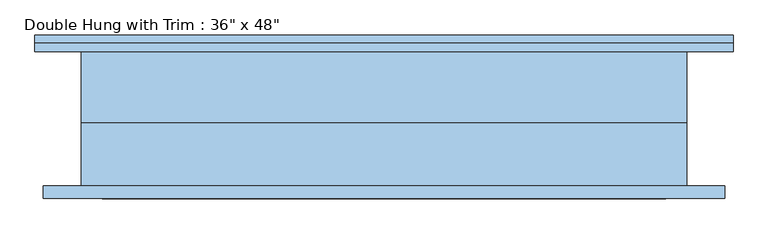
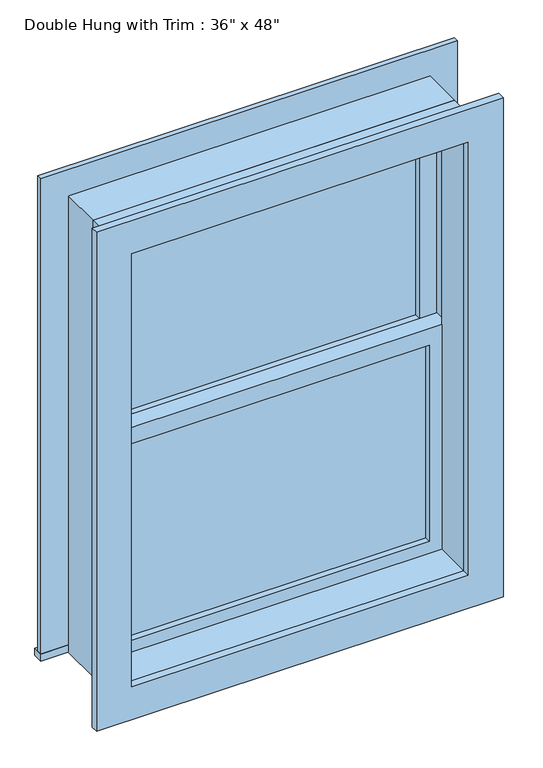
"""IFC4 building model written with IfcOpenShell, lengths in millimetres: window geometry."""

from ifc_helpers import new_model, si_unit, frame, origin, place, context, project, spatial, polyline, outline, extrude, source, transform, mapped, element, save


def window_31198920(model_context):
    return source(origin(), model_context, "Body", "SweptSolid", [
        extrude(outline(polyline([(-393.7, 22.225), (393.7, 22.225), (393.7, 9.525), (-393.7, 9.525), (-393.7, 22.225)])), frame((0.0, 0.0, 977.9), z_axis=(0.0, 0.0, 1.0), x_axis=(1.0, 0.0, 0.0)), (0.0, 0.0, 1.0), 523.875),
        extrude(outline(polyline([(1546.225, -438.15), (933.45, -438.15), (933.45, 438.15), (1546.225, 438.15), (1546.225, -438.15)]), holes=[polyline([(1501.775, -393.7), (1501.775, 393.7), (977.9, 393.7), (977.9, -393.7), (1501.775, -393.7)])]), frame((0.0, -6.35, 0.0), z_axis=(0.0, 1.0, 0.0), x_axis=(0.0, 0.0, 1.0)), (0.0, 0.0, 1.0), 44.45),
        extrude(outline(polyline([(-527.05, 127.0), (527.05, 127.0), (527.05, 101.6), (-527.05, 101.6), (-527.05, 127.0)])), frame((0.0, 0.0, 914.4), z_axis=(0.0, 0.0, 1.0), x_axis=(1.0, 0.0, 0.0)), (0.0, 0.0, 1.0), 19.05),
        extrude(outline(polyline([(2114.55, -438.15), (2114.55, 438.15), (933.45, 438.15), (933.45, 527.05), (2203.45, 527.05), (2203.45, -527.05), (933.45, -527.05), (933.45, -438.15), (2114.55, -438.15)])), frame((0.0, 101.6, 0.0), z_axis=(0.0, 1.0, 0.0), x_axis=(0.0, 0.0, 1.0)), (0.0, 0.0, 1.0), 12.7),
        extrude(outline(polyline([(2190.75, 514.35), (2190.75, -514.35), (857.25, -514.35), (857.25, 514.35), (2190.75, 514.35)]), holes=[polyline([(2101.85, 425.45), (946.15, 425.45), (946.15, -425.45), (2101.85, -425.45), (2101.85, 425.45)])]), frame((0.0, -120.65, 0.0), z_axis=(0.0, 1.0, 0.0), x_axis=(0.0, 0.0, 1.0)), (0.0, 0.0, 1.0), 19.05),
        extrude(outline(polyline([(393.7, 53.975), (-393.7, 53.975), (-393.7, 66.675), (393.7, 66.675), (393.7, 53.975)])), frame((0.0, 0.0, 1546.225), z_axis=(0.0, 0.0, 1.0), x_axis=(1.0, 0.0, 0.0)), (0.0, 0.0, 1.0), 523.875),
        extrude(outline(polyline([(2114.55, -438.15), (1501.775, -438.15), (1501.775, 438.15), (2114.55, 438.15), (2114.55, -438.15)]), holes=[polyline([(2070.1, -393.7), (2070.1, 393.7), (1546.225, 393.7), (1546.225, -393.7), (2070.1, -393.7)])]), frame((0.0, 38.1, 0.0), z_axis=(0.0, 1.0, 0.0), x_axis=(0.0, 0.0, 1.0)), (0.0, 0.0, 1.0), 44.45),
        extrude(outline(polyline([(2133.6, -457.2), (914.4, -457.2), (914.4, 457.2), (2133.6, 457.2), (2133.6, -457.2)]), holes=[polyline([(2101.85, -425.45), (2101.85, 425.45), (946.15, 425.45), (946.15, -425.45), (2101.85, -425.45)])]), frame((0.0, -101.6, 0.0), z_axis=(0.0, 1.0, 0.0), x_axis=(0.0, 0.0, 1.0)), (0.0, 0.0, 1.0), 95.25),
        extrude(outline(polyline([(2133.6, 457.2), (2133.6, -457.2), (914.4, -457.2), (914.4, 457.2), (2133.6, 457.2)]), holes=[polyline([(2114.55, 438.15), (933.45, 438.15), (933.45, -438.15), (2114.55, -438.15), (2114.55, 438.15)])]), frame((0.0, -6.35, 0.0), z_axis=(0.0, 1.0, 0.0), x_axis=(0.0, 0.0, 1.0)), (0.0, 0.0, 1.0), 107.95),
    ])


if __name__ == "__main__":
    model = new_model("IFC4")
    model_context = context("Model", 3, world=origin())
    ifc_project = project(units=[si_unit("LENGTHUNIT", "METRE", prefix="MILLI")], contexts=[model_context])
    site = spatial("IfcSite", under=ifc_project)
    building = spatial("IfcBuilding", under=site)
    placement = place(None, origin())
    window_shape = window_31198920(model_context)
    element("IfcWindow", 1, ObjectType="Double Hung with Trim : 36\" x 48\"", at=placement, inside=building, context=model_context, shape_type="MappedRepresentation", body=[
        mapped(window_shape, transform((0.0, 0.0, 0.0), x_axis=(1.0, 0.0, 0.0), y_axis=(0.0, 1.0, 0.0), z_axis=(0.0, 0.0, 1.0))),
    ])
    save(model, "model.ifc")

# Revit data of these elements
# Type "Double Hung with Trim : 36\" x 48\""
#   Type Mark = "16"
#   Construction Type Id = "GSP4R"
#   Assembly Code = "B2020100"
#   Analytic Construction = "1/8 in Pilkington single glazing"
#   Visual Light Transmittance = 0.9
#   Solar Heat Gain Coefficient = 0.78
#   Heat Transfer Coefficient (U) = 0.6496 BTU/(h·ft²·°F)
#   Height = 4' - 0"
#   Default Sill Height = 3' - 0"
#   Trim Projection - Ext. = 0' - 0 1/2"
#   Trim Projection - Int. = 0' - 0 3/4"
#   Trim Width - Exterior = 0' - 3 1/2"
#   Trim Width - Interior = 0' - 3 1/2"
#   Width = 3' - 0"
#   Window Inset = 0' - 0 3/4"
#   Define Thermal Properties by = 1
#   Glass Pane Material = Glass
#   Sash Material = Sash
#   Trim Exterior Material = Trim
#   Trim Interior Material = Trim
#   Wall Closure = (empty or 0)
# Element 1 (IfcWindow, "Double Hung with Trim : 36\" x 48\"")
#   Materials on its faces: "Sash", "Trim", "Glass"
# Materials
#   "Glass": class "Glass", colour RGB 0 128 192, transparency 0.75, Description = "Soda Lime Glass", Cost = 0
#   "Sash": class "Wood", colour RGB 224 178 126, transparency 0
#   "Trim": class "Wood", colour RGB 224 178 126, transparency 0
